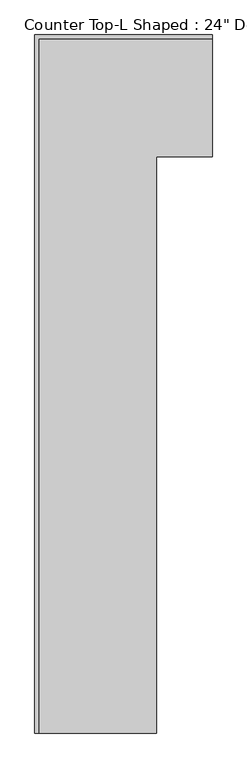
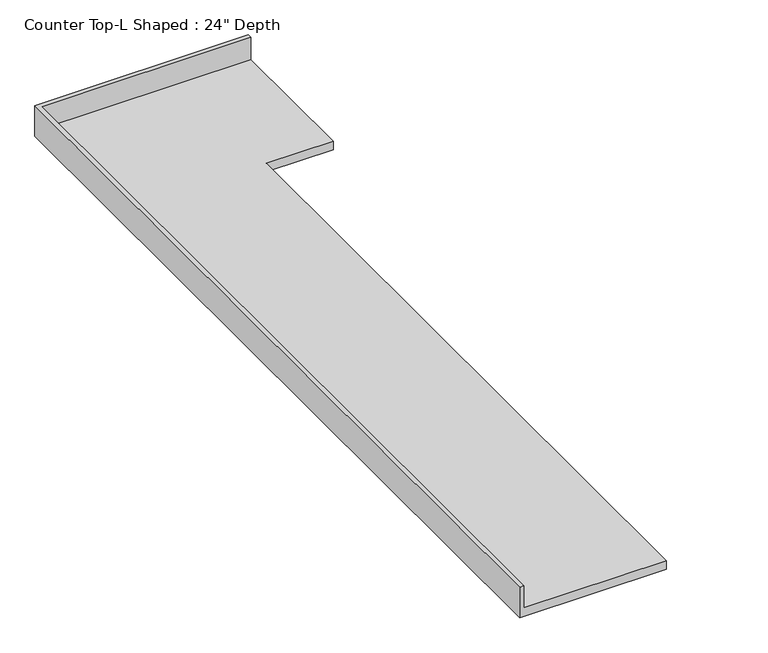
"""IFC4 building model written with IfcOpenShell, lengths in millimetres: furniture geometry."""

from ifc_helpers import new_model, si_unit, origin, place, context, project, spatial, faceted_brep, source, transform, mapped, element, save


def furniture_0681fcb1(model_context):
    return source(origin(), model_context, "Body", "Brep", [
        faceted_brep([(-565.4622951, -3632.2, 914.4), (-565.4622951, -635.0, 914.4), (-276.5372951, -635.0, 914.4), (-276.5372951, -19.05, 914.4), (-1181.4122951, -19.05, 914.4), (-1181.4122951, -3632.2, 914.4), (-276.5372951, 0.0, 876.3), (-276.5372951, -635.0, 876.3), (-565.4622951, -635.0, 876.3), (-565.4622951, -3632.2, 876.3), (-1200.4622951, -3632.2, 876.3), (-1200.4622951, 0.0, 876.3), (-1200.4622951, 0.0, 1016.0), (-276.5372951, 0.0, 1016.0), (-1200.4622951, -3632.2, 1016.0), (-1181.4122951, -3632.2, 1016.0), (-276.5372951, -19.05, 1016.0), (-1181.4122951, -19.05, 1016.0)], [[[0, 1, 2, 3, 4, 5]], [[6, 7, 8, 9, 10, 11]], [[6, 11, 12, 13]], [[11, 10, 14, 12]], [[14, 10, 9, 0, 5, 15]], [[1, 0, 9, 8]], [[2, 1, 8, 7]], [[7, 6, 13, 16, 3, 2]], [[12, 14, 15, 17, 16, 13]], [[3, 16, 17, 4]], [[17, 15, 5, 4]]]),
    ])


if __name__ == "__main__":
    model = new_model("IFC4")
    model_context = context("Model", 3, world=origin())
    ifc_project = project(units=[si_unit("LENGTHUNIT", "METRE", prefix="MILLI")], contexts=[model_context])
    site = spatial("IfcSite", under=ifc_project)
    building = spatial("IfcBuilding", under=site)
    placement = place(None, origin())
    furniture_shape = furniture_0681fcb1(model_context)
    element("IfcFurniture", 1, ObjectType="Counter Top-L Shaped : 24\" Depth", at=placement, inside=building, context=model_context, shape_type="MappedRepresentation", body=[
        mapped(furniture_shape, transform((0.0, 0.0, 0.0), x_axis=(1.0, 0.0, 0.0), y_axis=(0.0, 1.0, 0.0), z_axis=(0.0, 0.0, 1.0))),
    ])
    save(model, "model.ifc")

# Revit data of these elements
# Type "Counter Top-L Shaped : 24\" Depth"
#   Assembly Code = "C1030400"
#   Counter Thickness = 0' - 1 1/2"
#   Depth = 2' - 1"
#   Height = 3' - 0"
#   Length - Leg 1 [instance default] = 8' - 0"
#   Length - Leg 2 [instance default] = 6' - 0"
#   Counter Top Material = none
#   Default Elevation = 0
# Element 1 (IfcFurniture, "Counter Top-L Shaped : 24\" Depth")
#   Length - Leg 1 = 3' - 0 3/8"
#   Length - Leg 2 = 11' - 11"
#   Materials on its faces: "Counter Top"
# Materials
#   "Counter Top": class "Wood", colour RGB 226 177 128, transparency 0
